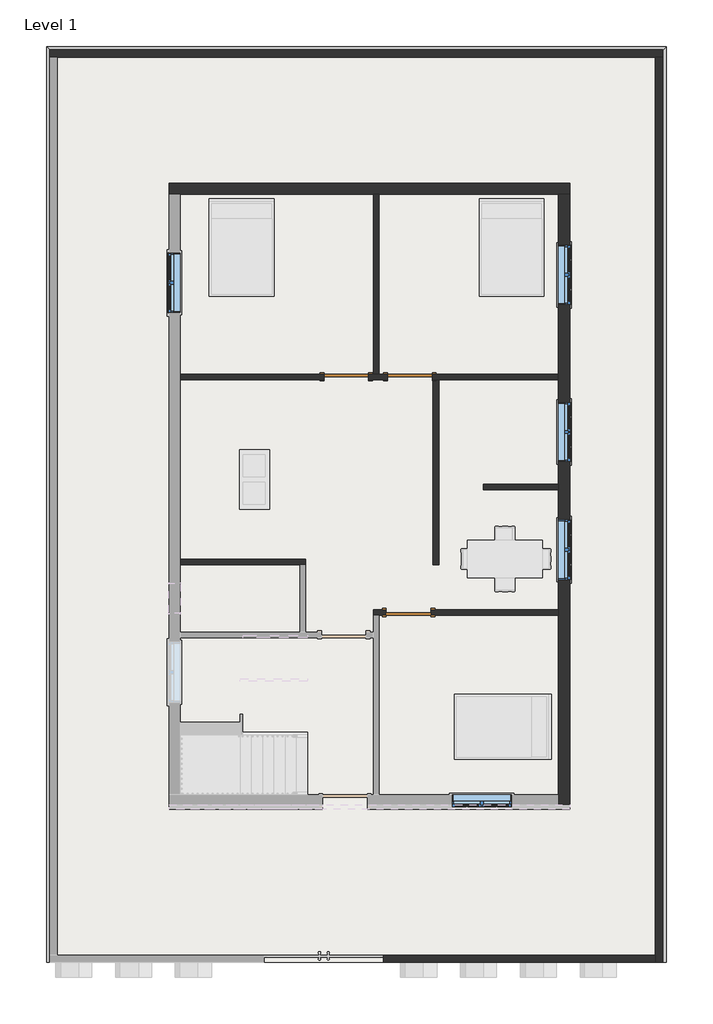
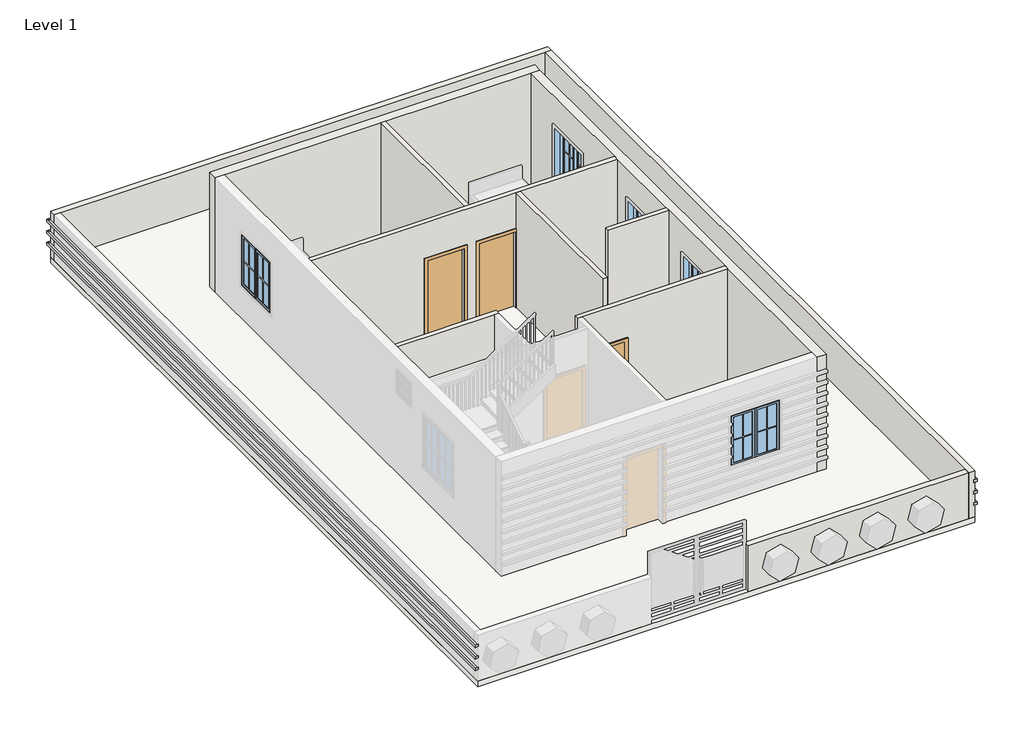
# One storey, part 2 of 4: 11 walls, 5 windows, 3 doors, 3 proxies, 1 slab.
"""IFC4 building model written with IfcOpenShell, lengths in millimetres."""

from ifc_helpers import new_model, si_unit, frame, origin, origin_with_axes, place, context, project, spatial, polyline, outline, extrude, faceted_brep, transform, mapped, element, save
from components import single_flush_door_3_17d80c48, single_flush_door_3_5e62189b, window_casement_double_window_4_576b2d2c

model = new_model("IFC4")

# Units and contexts
model_context = context("Model", 3, world=origin())
ifc_project = project(units=[si_unit("LENGTHUNIT", "METRE", prefix="MILLI")], contexts=[model_context])

# Site, building, storey
site = spatial("IfcSite", under=ifc_project)
building = spatial("IfcBuilding", under=site)
storey = spatial("IfcBuildingStorey", under=building, Name="Level 1", Elevation=0.0)

# Proxies
placement = place(None, origin())
element("IfcBuildingElementProxy", 1, Name="Reveal", ObjectType="Reveal", at=placement, inside=storey, context=model_context, shape_type="SweptSolid", body=[
    extrude(outline(polyline([(-7740.2753152, -9797.7989753), (-7832.3503152, -9797.7989753), (-7832.3503152, 8861.6760247), (-7740.2753152, 8769.6010247), (-7740.2753152, -9797.7989753)])), frame((0.0, 0.0, 304.8), z_axis=(0.0, 0.0, 1.0), x_axis=(1.0, 0.0, 0.0)), (0.0, 0.0, 1.0), 67.7333333),
    extrude(outline(polyline([(-7740.2753152, 8769.6010247), (-7832.3503152, 8861.6760247), (4797.7996848, 8861.6760247), (4705.7246848, 8769.6010247), (-7740.2753152, 8769.6010247)])), frame((0.0, 0.0, 304.8), z_axis=(0.0, 0.0, 1.0), x_axis=(1.0, 0.0, 0.0)), (0.0, 0.0, 1.0), 67.7333333),
    extrude(outline(polyline([(4705.7246848, 8769.6010247), (4797.7996848, 8861.6760247), (4797.7996848, -9797.7989753), (4705.7246848, -9797.7989753), (4705.7246848, 8769.6010247)])), frame((0.0, 0.0, 304.8), z_axis=(0.0, 0.0, 1.0), x_axis=(1.0, 0.0, 0.0)), (0.0, 0.0, 1.0), 67.7333333),
])
element("IfcBuildingElementProxy", 2, Name="Reveal", ObjectType="Reveal", at=placement, inside=storey, context=model_context, shape_type="SweptSolid", body=[
    extrude(outline(polyline([(-7740.2753152, -9797.7989753), (-7832.3503152, -9797.7989753), (-7832.3503152, 8861.6760247), (-7740.2753152, 8769.6010247), (-7740.2753152, -9797.7989753)])), frame((0.0, 0.0, 609.6), z_axis=(0.0, 0.0, 1.0), x_axis=(1.0, 0.0, 0.0)), (0.0, 0.0, 1.0), 67.7333333),
    extrude(outline(polyline([(-7740.2753152, 8769.6010247), (-7832.3503152, 8861.6760247), (4797.7996848, 8861.6760247), (4705.7246848, 8769.6010247), (-7740.2753152, 8769.6010247)])), frame((0.0, 0.0, 609.6), z_axis=(0.0, 0.0, 1.0), x_axis=(1.0, 0.0, 0.0)), (0.0, 0.0, 1.0), 67.7333333),
    extrude(outline(polyline([(4705.7246848, 8769.6010247), (4797.7996848, 8861.6760247), (4797.7996848, -9797.7989753), (4705.7246848, -9797.7989753), (4705.7246848, 8769.6010247)])), frame((0.0, 0.0, 609.6), z_axis=(0.0, 0.0, 1.0), x_axis=(1.0, 0.0, 0.0)), (0.0, 0.0, 1.0), 67.7333333),
])
element("IfcBuildingElementProxy", 3, Name="Reveal", ObjectType="Reveal", at=placement, inside=storey, context=model_context, shape_type="SweptSolid", body=[
    extrude(outline(polyline([(-7740.2753152, -9797.7989753), (-7832.3503152, -9797.7989753), (-7832.3503152, 8861.6760247), (-7740.2753152, 8769.6010247), (-7740.2753152, -9797.7989753)])), frame((0.0, 0.0, 914.4), z_axis=(0.0, 0.0, 1.0), x_axis=(1.0, 0.0, 0.0)), (0.0, 0.0, 1.0), 67.7333333),
    extrude(outline(polyline([(-7740.2753152, 8769.6010247), (-7832.3503152, 8861.6760247), (4797.7996848, 8861.6760247), (4705.7246848, 8769.6010247), (-7740.2753152, 8769.6010247)])), frame((0.0, 0.0, 914.4), z_axis=(0.0, 0.0, 1.0), x_axis=(1.0, 0.0, 0.0)), (0.0, 0.0, 1.0), 67.7333333),
    extrude(outline(polyline([(4705.7246848, 8769.6010247), (4797.7996848, 8861.6760247), (4797.7996848, -9797.7989753), (4705.7246848, -9797.7989753), (4705.7246848, 8769.6010247)])), frame((0.0, 0.0, 914.4), z_axis=(0.0, 0.0, 1.0), x_axis=(1.0, 0.0, 0.0)), (0.0, 0.0, 1.0), 67.7333333),
])

# Doors
single_flush_door_3_shape = single_flush_door_3_17d80c48(model_context)
element("IfcDoor", 4, ObjectType="Single-Flush : DOOR 3'", at=placement, inside=storey, context=model_context, shape_type="MappedRepresentation", body=[
    mapped(single_flush_door_3_shape, transform((-1721.4617403, 2133.1073441, 0.0), x_axis=(1.0, 0.0, 0.0), y_axis=(0.0, 1.0, 0.0), z_axis=(0.0, 0.0, 1.0))),
])
element("IfcDoor", 5, ObjectType="Single-Flush : DOOR 3'", at=placement, inside=storey, context=model_context, shape_type="MappedRepresentation", body=[
    mapped(single_flush_door_3_shape, transform((-451.4617403, -2667.4926559, 0.0), x_axis=(-1.0, 0.0, 0.0), y_axis=(0.0, -1.0, 0.0), z_axis=(0.0, 0.0, 1.0))),
])
single_flush_door_3_2_shape = single_flush_door_3_5e62189b(model_context)
element("IfcDoor", 6, ObjectType="Single-Flush : DOOR 3'", at=placement, inside=storey, context=model_context, shape_type="MappedRepresentation", body=[
    mapped(single_flush_door_3_2_shape, transform((-426.0617403, 2133.1073441, 0.0), x_axis=(-1.0, 0.0, 0.0), y_axis=(0.0, -1.0, 0.0), z_axis=(0.0, 0.0, 1.0))),
])

# Slab
element("IfcSlab", 7, ObjectType="FLOOR 6\"", at=placement, inside=storey, context=model_context, shape_type="SweptSolid", body=[
    extrude(outline(polyline([(4731.1246848, 8795.0010247), (4731.1246848, -9797.7989753), (-7765.6753152, -9797.7989753), (-7765.6753152, 8795.0010247), (4731.1246848, 8795.0010247)])), frame((0.0, 0.0, -152.4), z_axis=(0.0, 0.0, 1.0), x_axis=(1.0, 0.0, 0.0)), (0.0, 0.0, 1.0), 152.4),
])

# Walls
element("IfcWall", 8, ObjectType="ALL 4.5\"", at=placement, inside=storey, context=model_context, shape_type="Brep", body=[
    faceted_brep([(-1264.2617403, 2075.9573441, 0.0), (-883.2617403, 2075.9573441, 0.0), (-883.2617403, 2075.9573441, 2032.0), (31.1382597, 2075.9573441, 2032.0), (31.1382597, 2075.9573441, 0.0), (50.1882597, 2075.9573441, 0.0), (164.4882597, 2075.9573441, 0.0), (2602.8882597, 2075.9573441, 0.0), (2602.8882597, 2075.9573441, 3048.0), (164.4882597, 2075.9573441, 3048.0), (50.1882597, 2075.9573441, 3048.0), (-5106.0117403, 2075.9573441, 3048.0), (-5106.0117403, 2075.9573441, 0.0), (-2178.6617403, 2075.9573441, 0.0), (-2178.6617403, 2075.9573441, 2032.0), (-1264.2617403, 2075.9573441, 2032.0), (-883.2617403, 2190.2573441, 2032.0), (-883.2617403, 2190.2573441, 0.0), (-1054.7117403, 2190.2573441, 0.0), (-1169.0117403, 2190.2573441, 0.0), (-1264.2617403, 2190.2573441, 0.0), (-1264.2617403, 2190.2573441, 2032.0), (-2178.6617403, 2190.2573441, 2032.0), (-2178.6617403, 2190.2573441, 0.0), (-5106.0117403, 2190.2573441, 0.0), (-5106.0117403, 2190.2573441, 3048.0), (-1169.0117403, 2190.2573441, 3048.0), (-1054.7117403, 2190.2573441, 3048.0), (2602.8882597, 2190.2573441, 3048.0), (2602.8882597, 2190.2573441, 0.0), (31.1382597, 2190.2573441, 0.0), (31.1382597, 2190.2573441, 2032.0)], [[[0, 1, 2, 3, 4, 5, 6, 7, 8, 9, 10, 11, 12, 13, 14, 15]], [[16, 17, 18, 19, 20, 21, 22, 23, 24, 25, 26, 27, 28, 29, 30, 31]], [[13, 12, 24, 23]], [[30, 29, 7, 6, 5, 4]], [[20, 19, 18, 17, 1, 0]], [[8, 7, 29, 28]], [[12, 11, 25, 24]], [[21, 20, 0, 15]], [[22, 21, 15, 14]], [[23, 22, 14, 13]], [[2, 1, 17, 16]], [[3, 2, 16, 31]], [[4, 3, 31, 30]], [[11, 10, 9, 8, 28, 27, 26, 25]]]),
])
element("IfcWall", 9, ObjectType="ALL 4.5\"", at=placement, inside=storey, context=model_context, shape_type="SweptSolid", body=[
    extrude(outline(polyline([(50.1882597, -1695.9426559), (50.1882597, 2075.9573441), (164.4882597, 2075.9573441), (164.4882597, -1695.9426559), (50.1882597, -1695.9426559)])), origin_with_axes(), (0.0, 0.0, 1.0), 3048.0),
])
element("IfcWall", 10, ObjectType="ALL 4.5\"", at=placement, inside=storey, context=model_context, shape_type="SweptSolid", body=[
    extrude(outline(polyline([(1078.8882597, -57.6426559), (2602.8882597, -57.6426559), (2602.8882597, -171.9426559), (1078.8882597, -171.9426559), (1078.8882597, -57.6426559)])), origin_with_axes(), (0.0, 0.0, 1.0), 3048.0),
])
element("IfcWall", 11, ObjectType="ALL 4.5\"", at=placement, inside=storey, context=model_context, shape_type="Brep", body=[
    faceted_brep([(-908.6617403, -2610.3426559, 2032.0), (-908.6617403, -2610.3426559, 0.0), (-1169.0117403, -2610.3426559, 0.0), (-1169.0117403, -2610.3426559, 3048.0), (2602.8882597, -2610.3426559, 3048.0), (2602.8882597, -2610.3426559, 0.0), (5.7382597, -2610.3426559, 0.0), (5.7382597, -2610.3426559, 2032.0), (-1169.0117403, -2724.6426559, 0.0), (-1054.7117403, -2724.6426559, 0.0), (-908.6617403, -2724.6426559, 0.0), (-908.6617403, -2724.6426559, 2032.0), (5.7382597, -2724.6426559, 2032.0), (5.7382597, -2724.6426559, 0.0), (2602.8882597, -2724.6426559, 0.0), (2602.8882597, -2724.6426559, 3048.0), (-1054.7117403, -2724.6426559, 3048.0), (-1169.0117403, -2724.6426559, 3048.0)], [[[0, 1, 2, 3, 4, 5, 6, 7]], [[8, 9, 10, 11, 12, 13, 14, 15, 16, 17]], [[6, 5, 14, 13]], [[2, 1, 10, 9, 8]], [[5, 4, 15, 14]], [[3, 2, 8, 17]], [[11, 10, 1, 0]], [[12, 11, 0, 7]], [[13, 12, 7, 6]], [[4, 3, 17, 16, 15]]]),
])
element("IfcWall", 12, ObjectType="ALL 4.5\"", at=placement, inside=storey, context=model_context, shape_type="Brep", body=[
    faceted_brep([(-5106.0117403, -1695.9426559, 0.0), (-2667.6117403, -1695.9426559, 0.0), (-2553.3117403, -1695.9426559, 0.0), (-2553.3117403, -1695.9426559, 3048.0), (-2667.6117403, -1695.9426559, 3048.0), (-5106.0117403, -1695.9426559, 3048.0), (-5106.0117403, -1581.6426559, 0.0), (-5106.0117403, -1581.6426559, 3048.0), (-2553.3117403, -1581.6426559, 3048.0), (-2553.3117403, -1581.6426559, 0.0)], [[[0, 1, 2, 3, 4, 5]], [[6, 7, 8, 9]], [[2, 1, 0, 6, 9]], [[0, 5, 7, 6]], [[3, 2, 9, 8]], [[5, 4, 3, 8, 7]]]),
])
element("IfcWall", 13, ObjectType="ALL 4.5\"", at=placement, inside=storey, context=model_context, shape_type="SweptSolid", body=[
    extrude(outline(polyline([(-1169.0117403, 2190.2573441), (-1169.0117403, 5847.8573441), (-1054.7117403, 5847.8573441), (-1054.7117403, 2190.2573441), (-1169.0117403, 2190.2573441)])), origin_with_axes(), (0.0, 0.0, 1.0), 3048.0),
])
element("IfcWall", 14, ObjectType="CMD 6\"", at=placement, inside=storey, context=model_context, shape_type="Brep", body=[
    faceted_brep([(-7765.6753152, 8642.6010247, 0.0), (-7613.2753152, 8642.6010247, 0.0), (4578.7246848, 8642.6010247, 0.0), (4731.1246848, 8642.6010247, 0.0), (4731.1246848, 8642.6010247, 304.8), (4705.7246848, 8642.6010247, 304.8), (4705.7246848, 8642.6010247, 372.5333333), (4731.1246848, 8642.6010247, 372.5333333), (4731.1246848, 8642.6010247, 609.6), (4705.7246848, 8642.6010247, 609.6), (4705.7246848, 8642.6010247, 677.3333333), (4731.1246848, 8642.6010247, 677.3333333), (4731.1246848, 8642.6010247, 914.4), (4705.7246848, 8642.6010247, 914.4), (4705.7246848, 8642.6010247, 982.1333333), (4731.1246848, 8642.6010247, 982.1333333), (4731.1246848, 8642.6010247, 1219.2), (4578.7246848, 8642.6010247, 1219.2), (-7613.2753152, 8642.6010247, 1219.2), (-7765.6753152, 8642.6010247, 1219.2), (-7765.6753152, 8642.6010247, 982.1333333), (-7740.2753152, 8642.6010247, 982.1333333), (-7740.2753152, 8642.6010247, 914.4), (-7765.6753152, 8642.6010247, 914.4), (-7765.6753152, 8642.6010247, 677.3333333), (-7740.2753152, 8642.6010247, 677.3333333), (-7740.2753152, 8642.6010247, 609.6), (-7765.6753152, 8642.6010247, 609.6), (-7765.6753152, 8642.6010247, 372.5333333), (-7740.2753152, 8642.6010247, 372.5333333), (-7740.2753152, 8642.6010247, 304.8), (-7765.6753152, 8642.6010247, 304.8), (4731.1246848, 8795.0010247, 0.0), (-7765.6753152, 8795.0010247, 0.0), (-7765.6753152, 8795.0010247, 304.8), (4731.1246848, 8795.0010247, 304.8), (-7765.6753152, 8795.0010247, 1219.2), (4731.1246848, 8795.0010247, 1219.2), (4731.1246848, 8795.0010247, 982.1333333), (-7765.6753152, 8795.0010247, 982.1333333), (4731.1246848, 8795.0010247, 372.5333333), (-7765.6753152, 8795.0010247, 372.5333333), (-7765.6753152, 8795.0010247, 609.6), (4731.1246848, 8795.0010247, 609.6), (4731.1246848, 8795.0010247, 677.3333333), (-7765.6753152, 8795.0010247, 677.3333333), (-7765.6753152, 8795.0010247, 914.4), (4731.1246848, 8795.0010247, 914.4), (4705.7246848, 8769.6010247, 372.5333333), (-7740.2753152, 8769.6010247, 372.5333333), (-7740.2753152, 8769.6010247, 304.8), (4705.7246848, 8769.6010247, 304.8), (4705.7246848, 8769.6010247, 677.3333333), (-7740.2753152, 8769.6010247, 677.3333333), (-7740.2753152, 8769.6010247, 609.6), (4705.7246848, 8769.6010247, 609.6), (4705.7246848, 8769.6010247, 982.1333333), (-7740.2753152, 8769.6010247, 982.1333333), (-7740.2753152, 8769.6010247, 914.4), (4705.7246848, 8769.6010247, 914.4)], [[[0, 1, 2, 3, 4, 5, 6, 7, 8, 9, 10, 11, 12, 13, 14, 15, 16, 17, 18, 19, 20, 21, 22, 23, 24, 25, 26, 27, 28, 29, 30, 31]], [[32, 33, 34, 35]], [[36, 37, 38, 39]], [[40, 41, 42, 43]], [[44, 45, 46, 47]], [[3, 2, 1, 0, 33, 32]], [[19, 18, 17, 16, 37, 36]], [[3, 32, 35, 4]], [[37, 16, 15, 38]], [[7, 40, 43, 8]], [[11, 44, 47, 12]], [[19, 36, 39, 20]], [[33, 0, 31, 34]], [[41, 28, 27, 42]], [[45, 24, 23, 46]], [[48, 49, 29, 28, 41, 40, 7, 6]], [[50, 51, 5, 4, 35, 34, 31, 30]], [[49, 50, 30, 29]], [[49, 48, 51, 50]], [[51, 48, 6, 5]], [[52, 53, 25, 24, 45, 44, 11, 10]], [[54, 55, 9, 8, 43, 42, 27, 26]], [[53, 54, 26, 25]], [[53, 52, 55, 54]], [[55, 52, 10, 9]], [[56, 57, 21, 20, 39, 38, 15, 14]], [[58, 59, 13, 12, 47, 46, 23, 22]], [[57, 58, 22, 21]], [[57, 56, 59, 58]], [[59, 56, 14, 13]]]),
])
element("IfcWall", 15, ObjectType="CMD 6\"", at=placement, inside=storey, context=model_context, shape_type="Brep", body=[
    faceted_brep([(4578.7246848, 8642.6010247, 0.0), (4578.7246848, -9645.3989753, 0.0), (4578.7246848, -9797.7989753, 0.0), (4578.7246848, -9797.7989753, 1219.2), (4578.7246848, -9645.3989753, 1219.2), (4578.7246848, 8642.6010247, 1219.2), (4731.1246848, -9797.7989753, 0.0), (4731.1246848, 8642.6010247, 0.0), (4731.1246848, 8642.6010247, 304.8), (4731.1246848, -9797.7989753, 304.8), (4731.1246848, 8642.6010247, 1219.2), (4731.1246848, -9797.7989753, 1219.2), (4731.1246848, -9797.7989753, 982.1333333), (4731.1246848, 8642.6010247, 982.1333333), (4731.1246848, -9797.7989753, 372.5333333), (4731.1246848, 8642.6010247, 372.5333333), (4731.1246848, 8642.6010247, 609.6), (4731.1246848, -9797.7989753, 609.6), (4731.1246848, -9797.7989753, 677.3333333), (4731.1246848, 8642.6010247, 677.3333333), (4731.1246848, 8642.6010247, 914.4), (4731.1246848, -9797.7989753, 914.4), (4705.7246848, 8642.6010247, 982.1333333), (4705.7246848, 8642.6010247, 914.4), (4705.7246848, 8642.6010247, 677.3333333), (4705.7246848, 8642.6010247, 609.6), (4705.7246848, 8642.6010247, 372.5333333), (4705.7246848, 8642.6010247, 304.8), (4705.7246848, -9797.7989753, 304.8), (4705.7246848, -9797.7989753, 372.5333333), (4705.7246848, -9797.7989753, 609.6), (4705.7246848, -9797.7989753, 677.3333333), (4705.7246848, -9797.7989753, 914.4), (4705.7246848, -9797.7989753, 982.1333333)], [[[0, 1, 2, 3, 4, 5]], [[6, 7, 8, 9]], [[10, 11, 12, 13]], [[14, 15, 16, 17]], [[18, 19, 20, 21]], [[2, 1, 0, 7, 6]], [[5, 4, 3, 11, 10]], [[0, 5, 10, 13, 22, 23, 20, 19, 24, 25, 16, 15, 26, 27, 8, 7]], [[3, 2, 6, 9, 28, 29, 14, 17, 30, 31, 18, 21, 32, 33, 12, 11]], [[29, 26, 15, 14]], [[27, 28, 9, 8]], [[26, 29, 28, 27]], [[31, 24, 19, 18]], [[25, 30, 17, 16]], [[24, 31, 30, 25]], [[33, 22, 13, 12]], [[23, 32, 21, 20]], [[22, 33, 32, 23]]]),
])
element("IfcWall", 16, ObjectType="CMD 6\"", at=placement, inside=storey, context=model_context, shape_type="SweptSolid", body=[
    extrude(outline(polyline([(-958.4753152, -9645.3989753), (4578.7246848, -9645.3989753), (4578.7246848, -9797.7989753), (-958.4753152, -9797.7989753), (-958.4753152, -9645.3989753)])), origin_with_axes(), (0.0, 0.0, 1.0), 1219.2),
])
element("IfcWall", 17, ObjectType="WALL 9\"", at=placement, inside=storey, context=model_context, shape_type="Brep", body=[
    faceted_brep([(-5334.6117403, 5847.8573441, 0.0), (-5106.0117403, 5847.8573441, 0.0), (-1169.0117403, 5847.8573441, 0.0), (-1054.7117403, 5847.8573441, 0.0), (2602.8882597, 5847.8573441, 0.0), (2831.4882597, 5847.8573441, 0.0), (2831.4882597, 5847.8573441, 3048.0), (2602.8882597, 5847.8573441, 3048.0), (-1054.7117403, 5847.8573441, 3048.0), (-1169.0117403, 5847.8573441, 3048.0), (-5106.0117403, 5847.8573441, 3048.0), (-5334.6117403, 5847.8573441, 3048.0), (-5334.6117403, 6076.4573441, 0.0), (-5334.6117403, 6076.4573441, 3048.0), (2831.4882597, 6076.4573441, 3048.0), (2831.4882597, 6076.4573441, 0.0)], [[[0, 1, 2, 3, 4, 5, 6, 7, 8, 9, 10, 11]], [[12, 13, 14, 15]], [[5, 4, 3, 2, 1, 0, 12, 15]], [[6, 5, 15, 14]], [[0, 11, 13, 12]], [[11, 10, 9, 8, 7, 6, 14, 13]]]),
])
element("IfcWall", 18, ObjectType="WALL 9\"", at=placement, inside=storey, context=model_context, shape_type="Brep", body=[
    faceted_brep([(2602.8882597, 5847.8573441, 0.0), (2602.8882597, 2190.2573441, 0.0), (2602.8882597, 2075.9573441, 0.0), (2602.8882597, -57.6426559, 0.0), (2602.8882597, -171.9426559, 0.0), (2602.8882597, -2610.3426559, 0.0), (2602.8882597, -2724.6426559, 0.0), (2602.8882597, -6382.2426559, 0.0), (2602.8882597, -6610.8426559, 0.0), (2602.8882597, -6610.8426559, 304.8), (2602.8882597, -6585.4426559, 304.8), (2602.8882597, -6585.4426559, 372.5333333), (2602.8882597, -6610.8426559, 372.5333333), (2602.8882597, -6610.8426559, 591.2994231), (2602.8882597, -6585.4426559, 591.2994231), (2602.8882597, -6585.4426559, 659.0327564), (2602.8882597, -6610.8426559, 659.0327564), (2602.8882597, -6610.8426559, 877.7988461), (2602.8882597, -6585.4426559, 877.7988461), (2602.8882597, -6585.4426559, 945.5321795), (2602.8882597, -6610.8426559, 945.5321795), (2602.8882597, -6610.8426559, 1164.2982692), (2602.8882597, -6585.4426559, 1164.2982692), (2602.8882597, -6585.4426559, 1232.0316025), (2602.8882597, -6610.8426559, 1232.0316025), (2602.8882597, -6610.8426559, 1450.7976923), (2602.8882597, -6585.4426559, 1450.7976923), (2602.8882597, -6585.4426559, 1518.5310256), (2602.8882597, -6610.8426559, 1518.5310256), (2602.8882597, -6610.8426559, 1737.2971154), (2602.8882597, -6585.4426559, 1737.2971154), (2602.8882597, -6585.4426559, 1805.0304487), (2602.8882597, -6610.8426559, 1805.0304487), (2602.8882597, -6610.8426559, 2023.7965384), (2602.8882597, -6585.4426559, 2023.7965384), (2602.8882597, -6585.4426559, 2091.5298718), (2602.8882597, -6610.8426559, 2091.5298718), (2602.8882597, -6610.8426559, 2310.2959615), (2602.8882597, -6585.4426559, 2310.2959615), (2602.8882597, -6585.4426559, 2378.0292948), (2602.8882597, -6610.8426559, 2378.0292948), (2602.8882597, -6610.8426559, 2596.7953846), (2602.8882597, -6585.4426559, 2596.7953846), (2602.8882597, -6585.4426559, 2664.5287179), (2602.8882597, -6610.8426559, 2664.5287179), (2602.8882597, -6610.8426559, 3048.0), (2602.8882597, -6382.2426559, 3048.0), (2602.8882597, -2724.6426559, 3048.0), (2602.8882597, -2610.3426559, 3048.0), (2602.8882597, -171.9426559, 3048.0), (2602.8882597, -57.6426559, 3048.0), (2602.8882597, 2075.9573441, 3048.0), (2602.8882597, 2190.2573441, 3048.0), (2602.8882597, 5847.8573441, 3048.0), (2602.8882597, 3599.9573441, 2260.6), (2602.8882597, 3599.9573441, 914.4), (2602.8882597, 4819.1573441, 914.4), (2602.8882597, 4819.1573441, 2260.6), (2602.8882597, 399.5573441, 2260.6), (2602.8882597, 399.5573441, 914.4), (2602.8882597, 1618.7573441, 914.4), (2602.8882597, 1618.7573441, 2260.6), (2602.8882597, -2000.7426559, 2260.6), (2602.8882597, -2000.7426559, 914.4), (2602.8882597, -781.5426559, 914.4), (2602.8882597, -781.5426559, 2260.6), (2831.4882597, -6610.8426559, 0.0), (2831.4882597, 5847.8573441, 0.0), (2831.4882597, 5847.8573441, 3048.0), (2831.4882597, -6610.8426559, 3048.0), (2831.4882597, -6610.8426559, 2664.5287179), (2831.4882597, -6585.4426559, 2664.5287179), (2831.4882597, -6585.4426559, 2596.7953846), (2831.4882597, -6610.8426559, 2596.7953846), (2831.4882597, -6610.8426559, 2378.0292948), (2831.4882597, -6585.4426559, 2378.0292948), (2831.4882597, -6585.4426559, 2310.2959615), (2831.4882597, -6610.8426559, 2310.2959615), (2831.4882597, -6610.8426559, 2091.5298718), (2831.4882597, -6585.4426559, 2091.5298718), (2831.4882597, -6585.4426559, 2023.7965384), (2831.4882597, -6610.8426559, 2023.7965384), (2831.4882597, -6610.8426559, 1805.0304487), (2831.4882597, -6585.4426559, 1805.0304487), (2831.4882597, -6585.4426559, 1737.2971154), (2831.4882597, -6610.8426559, 1737.2971154), (2831.4882597, -6610.8426559, 1518.5310256), (2831.4882597, -6585.4426559, 1518.5310256), (2831.4882597, -6585.4426559, 1450.7976923), (2831.4882597, -6610.8426559, 1450.7976923), (2831.4882597, -6610.8426559, 1232.0316025), (2831.4882597, -6585.4426559, 1232.0316025), (2831.4882597, -6585.4426559, 1164.2982692), (2831.4882597, -6610.8426559, 1164.2982692), (2831.4882597, -6610.8426559, 945.5321795), (2831.4882597, -6585.4426559, 945.5321795), (2831.4882597, -6585.4426559, 877.7988461), (2831.4882597, -6610.8426559, 877.7988461), (2831.4882597, -6610.8426559, 659.0327564), (2831.4882597, -6585.4426559, 659.0327564), (2831.4882597, -6585.4426559, 591.2994231), (2831.4882597, -6610.8426559, 591.2994231), (2831.4882597, -6610.8426559, 372.5333333), (2831.4882597, -6585.4426559, 372.5333333), (2831.4882597, -6585.4426559, 304.8), (2831.4882597, -6610.8426559, 304.8), (2831.4882597, 3599.9573441, 914.4), (2831.4882597, 3599.9573441, 2260.6), (2831.4882597, 4819.1573441, 2260.6), (2831.4882597, 4819.1573441, 914.4), (2831.4882597, 399.5573441, 914.4), (2831.4882597, 399.5573441, 2260.6), (2831.4882597, 1618.7573441, 2260.6), (2831.4882597, 1618.7573441, 914.4), (2831.4882597, -2000.7426559, 914.4), (2831.4882597, -2000.7426559, 2260.6), (2831.4882597, -781.5426559, 2260.6), (2831.4882597, -781.5426559, 914.4)], [[[0, 1, 2, 3, 4, 5, 6, 7, 8, 9, 10, 11, 12, 13, 14, 15, 16, 17, 18, 19, 20, 21, 22, 23, 24, 25, 26, 27, 28, 29, 30, 31, 32, 33, 34, 35, 36, 37, 38, 39, 40, 41, 42, 43, 44, 45, 46, 47, 48, 49, 50, 51, 52, 53], [54, 55, 56, 57], [58, 59, 60, 61], [62, 63, 64, 65]], [[66, 67, 68, 69, 70, 71, 72, 73, 74, 75, 76, 77, 78, 79, 80, 81, 82, 83, 84, 85, 86, 87, 88, 89, 90, 91, 92, 93, 94, 95, 96, 97, 98, 99, 100, 101, 102, 103, 104, 105], [106, 107, 108, 109], [110, 111, 112, 113], [114, 115, 116, 117]], [[8, 7, 6, 5, 4, 3, 2, 1, 0, 67, 66]], [[0, 53, 68, 67]], [[8, 66, 105, 9]], [[69, 45, 44, 70]], [[12, 102, 101, 13]], [[16, 98, 97, 17]], [[20, 94, 93, 21]], [[24, 90, 89, 25]], [[28, 86, 85, 29]], [[32, 82, 81, 33]], [[36, 78, 77, 37]], [[40, 74, 73, 41]], [[55, 54, 107, 106]], [[56, 55, 106, 109]], [[57, 56, 109, 108]], [[54, 57, 108, 107]], [[59, 58, 111, 110]], [[60, 59, 110, 113]], [[61, 60, 113, 112]], [[58, 61, 112, 111]], [[63, 62, 115, 114]], [[64, 63, 114, 117]], [[65, 64, 117, 116]], [[62, 65, 116, 115]], [[53, 52, 51, 50, 49, 48, 47, 46, 45, 69, 68]], [[11, 103, 102, 12]], [[104, 10, 9, 105]], [[103, 11, 10, 104]], [[15, 99, 98, 16]], [[100, 14, 13, 101]], [[99, 15, 14, 100]], [[19, 95, 94, 20]], [[96, 18, 17, 97]], [[95, 19, 18, 96]], [[23, 91, 90, 24]], [[92, 22, 21, 93]], [[91, 23, 22, 92]], [[27, 87, 86, 28]], [[88, 26, 25, 89]], [[87, 27, 26, 88]], [[31, 83, 82, 32]], [[84, 30, 29, 85]], [[83, 31, 30, 84]], [[35, 79, 78, 36]], [[80, 34, 33, 81]], [[79, 35, 34, 80]], [[39, 75, 74, 40]], [[76, 38, 37, 77]], [[75, 39, 38, 76]], [[43, 71, 70, 44]], [[72, 42, 41, 73]], [[71, 43, 42, 72]]]),
])

# Windows
window_casement_double_window_4_shape = window_casement_double_window_4_576b2d2c(model_context)
element("IfcWindow", 19, ObjectType="Window-Casement-Double : WINDOW 4'", at=placement, inside=storey, context=model_context, shape_type="MappedRepresentation", body=[
    mapped(window_casement_double_window_4_shape, transform((-5220.3117403, 4047.6323441, 0.0), x_axis=(0.0, 1.0, 0.0), y_axis=(-1.0, 0.0, 0.0), z_axis=(0.0, 0.0, 1.0))),
])
element("IfcWindow", 20, ObjectType="Window-Casement-Double : WINDOW 4'", at=placement, inside=storey, context=model_context, shape_type="MappedRepresentation", body=[
    mapped(window_casement_double_window_4_shape, transform((2717.1882597, 4209.5573441, 0.0), x_axis=(0.0, -1.0, 0.0), y_axis=(1.0, 0.0, 0.0), z_axis=(0.0, 0.0, 1.0))),
])
element("IfcWindow", 21, ObjectType="Window-Casement-Double : WINDOW 4'", at=placement, inside=storey, context=model_context, shape_type="MappedRepresentation", body=[
    mapped(window_casement_double_window_4_shape, transform((2717.1882597, 1009.1573441, 0.0), x_axis=(0.0, -1.0, 0.0), y_axis=(1.0, 0.0, 0.0), z_axis=(0.0, 0.0, 1.0))),
])
element("IfcWindow", 22, ObjectType="Window-Casement-Double : WINDOW 4'", at=placement, inside=storey, context=model_context, shape_type="MappedRepresentation", body=[
    mapped(window_casement_double_window_4_shape, transform((2717.1882597, -1391.1426559, 0.0), x_axis=(0.0, -1.0, 0.0), y_axis=(1.0, 0.0, 0.0), z_axis=(0.0, 0.0, 1.0))),
])
element("IfcWindow", 23, ObjectType="Window-Casement-Double : WINDOW 4'", at=placement, inside=storey, context=model_context, shape_type="MappedRepresentation", body=[
    mapped(window_casement_double_window_4_shape, transform((1040.7882597, -6496.5426559, 0.0), x_axis=(-1.0, 0.0, 0.0), y_axis=(0.0, -1.0, 0.0), z_axis=(0.0, 0.0, 1.0))),
])

save(model, "model.ifc")

# Revit data of these elements
# Type "Single-Flush : DOOR 3'"
#   Type Mark = "8"
#   Construction Type Id = "MDOOR"
#   Assembly Code = "C1020"
#   Analytic Construction = "Metal"
#   Thickness = 0' - 2"
#   Heat Transfer Coefficient (U) = 0.651978 BTU/(h·ft²·°F)
#   Height = 6' - 8"
#   Trim Projection Ext = 0' - 1"
#   Trim Projection Int = 0' - 1"
#   Trim Width = 0' - 3"
#   Width = 3' - 0"
#   Define Thermal Properties by = 1
#   Door Material = Door - Panel
#   Frame Material = Door - Frame
#   Visual Light Transmittance = 0
#   Solar Heat Gain Coefficient = 0
#   Function = (empty or 0)
#   Wall Closure = (empty or 0)
# Type "FLOOR 6\""
#   Assembly Code = "B1010"
#   Function = 0
#   Layers, outside or top first: 0' - 6" no material (function 1)
# Type "ALL 4.5\""
#   Assembly Code = "B2010"
#   Layers, outside or top first: 0' - 4 1/2" no material (function 1)
# Type "CMD 6\""
#   Assembly Code = "B2010"
#   Layers, outside or top first: 0' - 6" "Carpet (1)" (function 1)
# Type "WALL 9\""
#   Assembly Code = "B2010"
#   Layers, outside or top first: 0' - 9" "Carpet (1)" (function 1)
# Type "Window-Casement-Double : WINDOW 4'"
#   Type Mark = "18"
#   Fire Rating = "0.5h"
#   Assembly Code = "B2020100"
#   Analytic Construction = "Double glazing - domestic"
#   Frame Extension [instance default] = 0' - 0 1/4"
#   Window Inset [instance default] = 0' - 0"
#   Wall Thickness [instance default] = 0' - 6"
#   Interior Wall Closure [instance default] = 0' - 2 1/4"
#   Half Width = 2' - 0"
#   Visual Light Transmittance = 0.81
#   Thermal Resistance (R) = 1.8146 (h·ft²·°F)/BTU
#   Solar Heat Gain Coefficient = 0.76
#   Rough Width = 4' - 0 1/2"
#   Rough Height = 4' - 5 1/2"
#   Height = 4' - 5"
#   Heat Transfer Coefficient (U) = 0.5511 BTU/(h·ft²·°F)
#   Exterior Wall Closure [instance default] = 0' - 1 1/4"
#   Extension Jamb [instance default] = 0' - 2 1/4"
#   Default Sill Height = 3' - 0"
#   Width = 4' - 0"
#   Muntin Visibility = yes
#   Interior Trim Visibility [instance default] = yes
#   Exterior Trim Visibility [instance default] = yes
#   Extension Jamb Visibility [instance default] = yes
#   Interior Trim Material = Wood - Stained
#   Muntin Pattern = Muntin Pattern_2x2 : Muntin Pattern_2x2
#   Interior Trim = Trim-Window-Interior-Flat : Picture Frame
#   Interior Frame Material = Wood - Stained
#   Glass Panel Material = Glass
#   Exterior Trim Material = Clad - White
#   Exterior Trim = Trim-Window-Exterior-Flat : with Sill
#   Exterior Frame Material = Clad - White
#   Wall Closure = (empty or 0)
# Elements 4, 5, 6 (IfcDoor, "Single-Flush : DOOR 3'")
#   Phase Created = New Construction
#   Materials on its faces: "Door - Frame", "Door - Panel"
# Element 7 (IfcSlab, "FLOOR 6\"")
#   Height Offset From Level = 0' - 0"
#   Phase Created = New Construction
#   Materials on its faces: "Door - Frame", "Default Floor", "bed frame"
# Elements 8, 9, 10, 12, 13 (IfcWall, "ALL 4.5\"")
#   Top Offset = 0' - 0"
#   Base Offset = 0' - 0"
#   Unconnected Height = 10' - 0"
#   wall height = 10' - 0"
#   Phase Created = New Construction
#   Base Constraint = Level 1
#   Materials on its faces: "Default Wall"
# Element 11 (IfcWall, "ALL 4.5\"")
#   Top Offset = 0' - 0"
#   Base Offset = 0' - 0"
#   Unconnected Height = 10' - 0"
#   wall height = 10' - 0"
#   Phase Created = New Construction
#   Base Constraint = Level 1
#   Materials on its faces: "Default Wall", "Clad - White"
# Elements 14, 15, 16 (IfcWall, "CMD 6\"")
#   Top Offset = 0' - 0"
#   Base Offset = 0' - 0"
#   Unconnected Height = 4' - 0"
#   wall height = 4' - 0"
#   Phase Created = New Construction
#   Base Constraint = Level 1
#   Materials on its faces: "Carpet (1)", "Door - Frame"
# Elements 17, 18 (IfcWall, "WALL 9\"")
#   Top Offset = 0' - 0"
#   Base Offset = 0' - 0"
#   Unconnected Height = 10' - 0"
#   wall height = 10' - 0"
#   Phase Created = New Construction
#   Base Constraint = Level 1
#   Materials on its faces: "Carpet (1)", "Wood - Stained"
# Element 19 (IfcWindow, "Window-Casement-Double : WINDOW 4'")
#   Mark = "2"
#   Window Inset = 0' - 0"
#   Interior Wall Closure = 0' - 2 1/4"
#   Frame Extension = 0' - 0 1/4"
#   Exterior Wall Closure = 0' - 1 1/4"
#   Interior Trim Visibility = yes
#   Exterior Trim Visibility = yes
#   Phase Created = New Construction
#   Materials on its faces: "Wood - Stained", "Glass", "Clad - White"
# Element 20 (IfcWindow, "Window-Casement-Double : WINDOW 4'")
#   Mark = "3"
#   Window Inset = 0' - 0"
#   Interior Wall Closure = 0' - 2 1/4"
#   Frame Extension = 0' - 0 1/4"
#   Exterior Wall Closure = 0' - 1 1/4"
#   Interior Trim Visibility = yes
#   Exterior Trim Visibility = yes
#   Phase Created = New Construction
#   Materials on its faces: "Wood - Stained", "Glass", "Clad - White"
# Element 21 (IfcWindow, "Window-Casement-Double : WINDOW 4'")
#   Mark = "4"
#   Window Inset = 0' - 0"
#   Interior Wall Closure = 0' - 2 1/4"
#   Frame Extension = 0' - 0 1/4"
#   Exterior Wall Closure = 0' - 1 1/4"
#   Interior Trim Visibility = yes
#   Exterior Trim Visibility = yes
#   Phase Created = New Construction
#   Materials on its faces: "Wood - Stained", "Glass", "Clad - White"
# Element 22 (IfcWindow, "Window-Casement-Double : WINDOW 4'")
#   Mark = "5"
#   Window Inset = 0' - 0"
#   Interior Wall Closure = 0' - 2 1/4"
#   Frame Extension = 0' - 0 1/4"
#   Exterior Wall Closure = 0' - 1 1/4"
#   Interior Trim Visibility = yes
#   Exterior Trim Visibility = yes
#   Phase Created = New Construction
#   Materials on its faces: "Wood - Stained", "Glass", "Clad - White"
# Element 23 (IfcWindow, "Window-Casement-Double : WINDOW 4'")
#   Mark = "6"
#   Window Inset = 0' - 0"
#   Interior Wall Closure = 0' - 2 1/4"
#   Frame Extension = 0' - 0 1/4"
#   Exterior Wall Closure = 0' - 1 1/4"
#   Interior Trim Visibility = yes
#   Exterior Trim Visibility = yes
#   Phase Created = New Construction
#   Materials on its faces: "Wood - Stained", "Glass", "Clad - White"
# Materials
#   "Door - Panel": class "Wood", colour RGB 210 159 95, transparency 0, Cost = 0
#   "Door - Frame": colour RGB 118 70 51, transparency 0, Cost = 0
#   "Carpet (1)": class "Carpet", colour RGB 124 80 67, transparency 0, Description = "Interior finish", Cost = 0
#   "Wood - Stained": class "Wood", colour RGB 224 178 126, transparency 0, Cost = 0
#   "Glass": class "Glass", colour RGB 0 128 192, transparency 0.75, Description = "Soda Lime Glass", Cost = 0
#   "Clad - White": class "Wood", colour RGB 242 242 238, transparency 0, Cost = 0
#   "Default Floor": colour RGB 128 128 128, transparency 0, Cost = 0
#   "bed frame": colour RGB 90 73 37, transparency 0, Cost = 0
#   "Default Wall": colour RGB 128 128 128, transparency 0, Cost = 0
